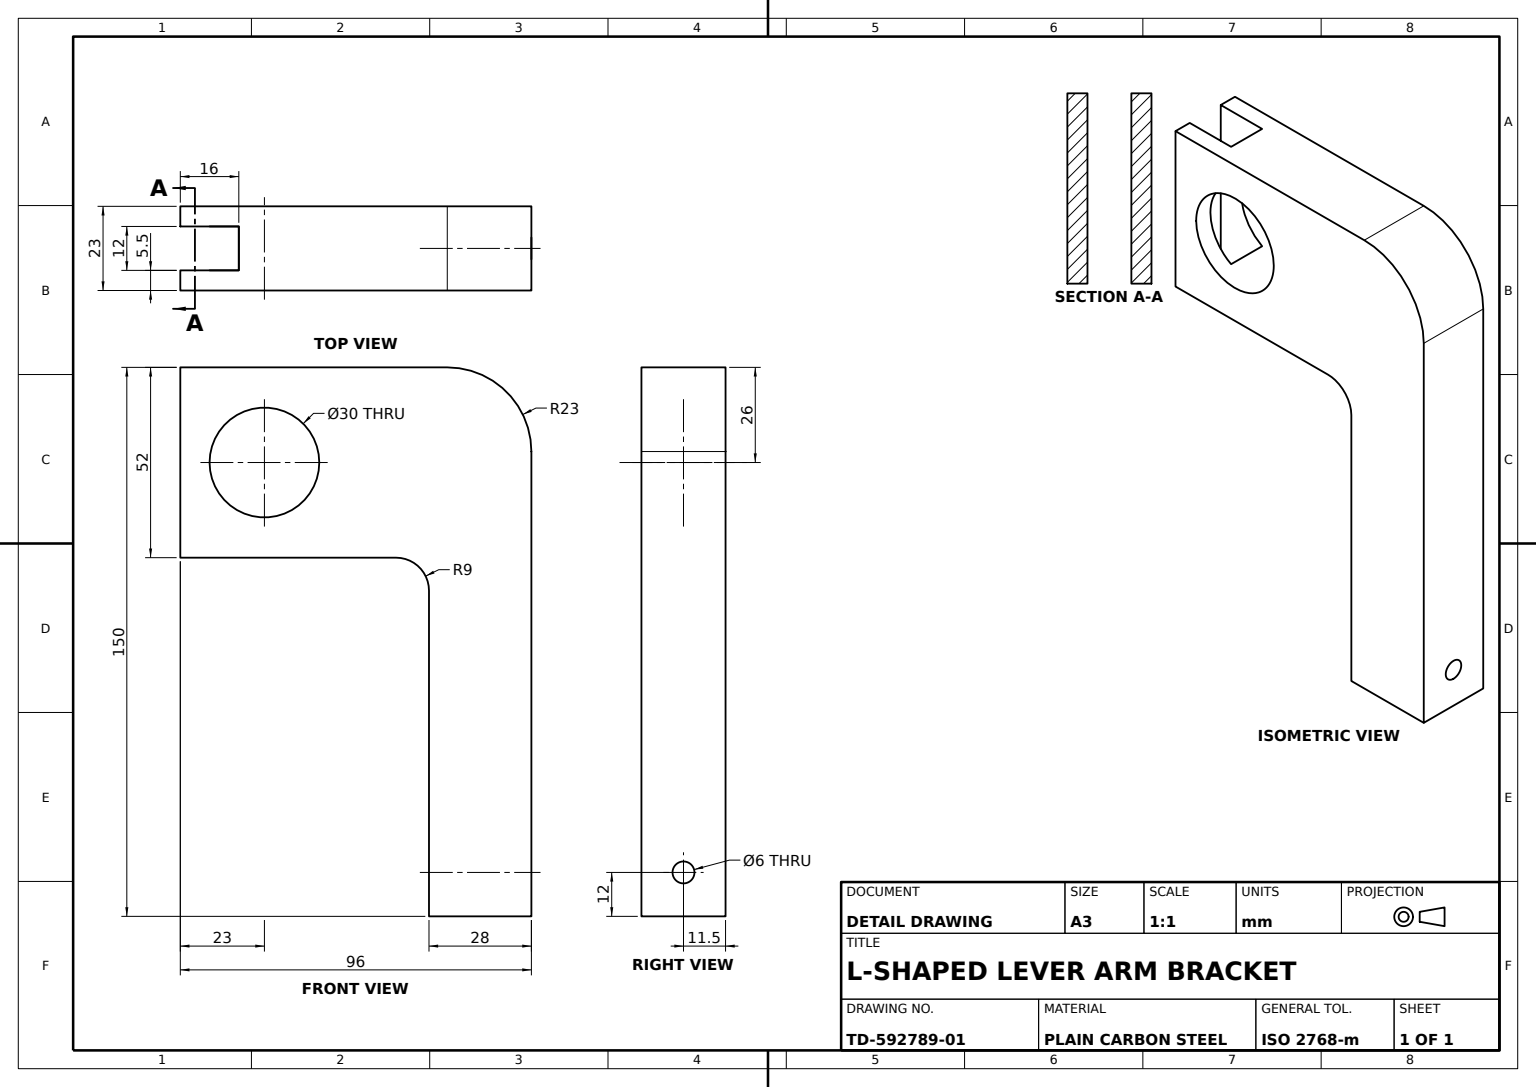
SolidWorks part; units mm, degrees
material "Plain Carbon Steel"
ref_plane "Front Plane" through (0, 0, 0) normal (0, 0, 1) x (1, 0, 0)
ref_plane "Top Plane" through (0, 0, 0) normal (0, 1, 0) x (1, 0, 0)
ref_plane "Right Plane" through (0, 0, 0) normal (1, 0, 0) x (0, 0, -1)
sketch "Bracket Profile Sketch" plane through (0, 0, 0) normal (0, 0, 1) x (1, 0, 0)
  line L0 (-23, -26) -> (-23, 26)
  line L1 (-23, 26) -> (50, 26)
  line L2 (73, 3) -> (73, -124)
  line L3 (73, -124) -> (45, -124)
  line L4 (45, -124) -> (45, -35)
  line L5 (36, -26) -> (-23, -26)
  circle A0 centre (0, 0) radius 6
  circle A1 centre (0, 0) radius 15
  arc A2 (45, -35) -> (36, -26) centre (36, -35) ccw
  arc A3 (73, 3) -> (50, 26) centre (50, 3) ccw
  point P7 (-23, 0)
  point P15 (73, 26)
  dimension "D1" = 12
  dimension "D2" = 30
  dimension "D9" = 9
  dimension "D10" = 23
  dimension "D3" = 23
  dimension "D4" = 52
  dimension "D5" = 26
  dimension "D6" = 96
  dimension "D7" = 150
  dimension "D8" = 28
extrude "L-Bracket Body" add sketch "Bracket Profile Sketch" along normal mid plane 23 contours L2 A3 L1 L0 L5 A2 L4 L3 A1
sketch "Slot Cut Sketch" plane through (0, 26, 0) normal (0, 1, 0) x (1, 0, 0)
  line L0 (-23, -11.5) -> (-23, 11.5) construction
  line L1 (-23, 6) -> (-7, 6)
  line L2 (-23, 6) -> (-23, -6)
  line L3 (-23, -6) -> (-7, -6)
  line L4 (-7, 6) -> (-7, -6)
  dimension "D1" = 12
  dimension "D2" = 6
  dimension "D3" = 16
extrude "Slot Cut" cut sketch "Slot Cut Sketch" against normal blind 63
sketch "End Hole Sketch" plane through (73, 0, 0) normal (1, 0, 0) x (0, 0, -1)
  line L0 (-11.5, -124) -> (11.5, -124) construction
  line L2 (11.5, 3) -> (11.5, -124) construction
  circle A0 centre (0, -112) radius 3
  dimension "D2" = 6
  dimension "D1" = 12
  dimension "D3" = 11.5
extrude "End Hole" cut sketch "End Hole Sketch" against normal blind 63
